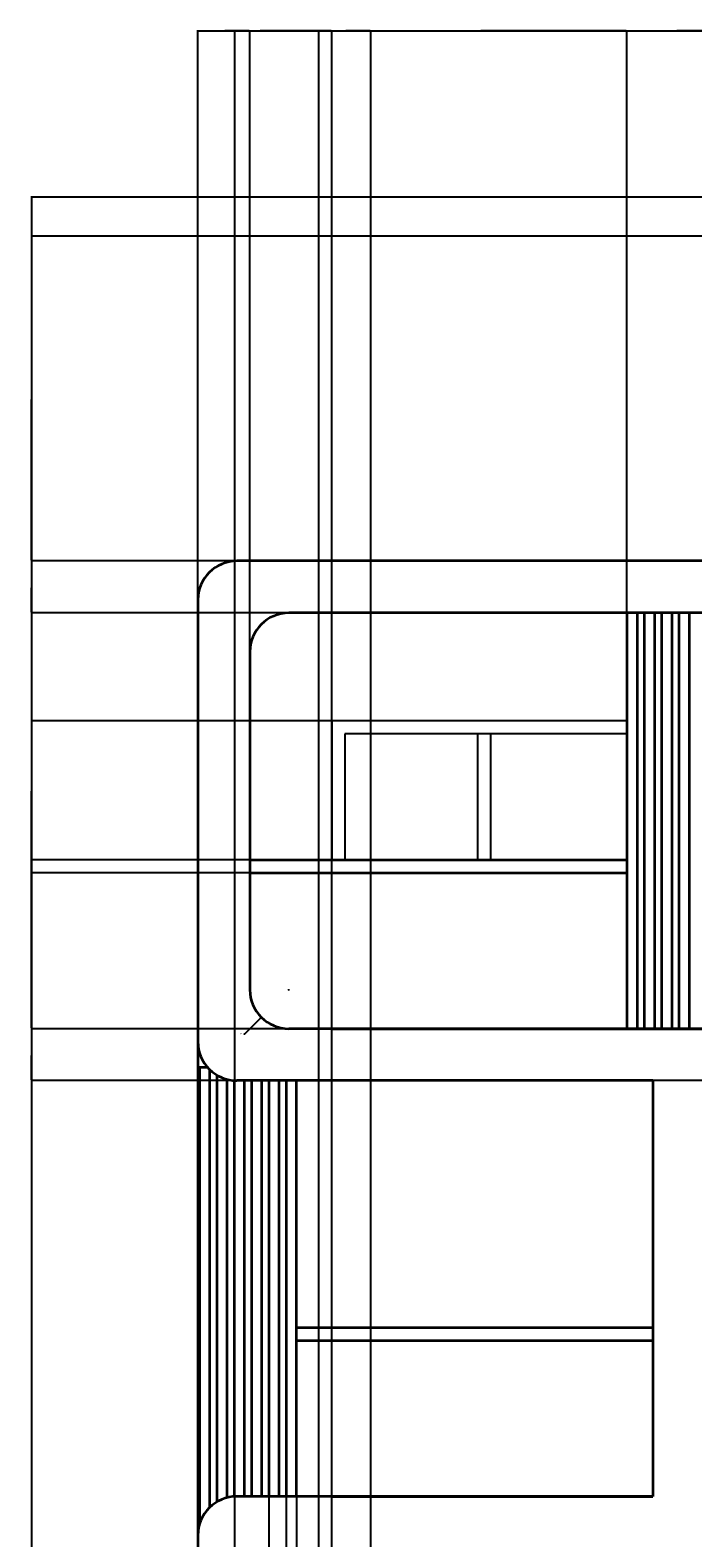
# Model space of a CAD drawing. Units: inches. Extents: x -15 to 605, y -220 to 570.
# Tile 7 of 10: x -15 to 138, y 222 to 570. Entities that reach past the tile are written whole.
import ezdxf

# ---------------------------------------------------------------- set-up
doc = ezdxf.new("R2010")
doc.units = ezdxf.units.IN
doc.header["$MEASUREMENT"] = 0
for name, color, linetype, lineweight in [('A-ANNO-DIMS', 2, 'Continuous', 18), ('A-ELEV', 7, 'Continuous', 35), ('A-GLAZ', 4, 'Continuous', 25)]:
    doc.layers.add(name, color=color, linetype=linetype, lineweight=lineweight)
doc.styles.get("Standard").update_dxf_attribs({"font": 'arial.ttf'})
doc.dimstyles.get("Standard").update_dxf_attribs({"dimtxt": 0.18, "dimasz": 0.18, "dimexe": 0.18, "dimexo": 0.0625, "dimgap": 0.09, "dimtad": 0, "dimtih": 1, "dimtoh": 1, "dimdec": 4, "dimzin": 0, "dimdsep": 46, "dimtxsty": 'Standard', "dimcen": 0.09, "dimadec": 0, "dimazin": 0, "dimtfac": 1, "dimtdec": 4, "dimtofl": 0, "dimtmove": 0, "dimatfit": 3, "dimfxl": 1, "dimtolj": 1, "dimtzin": 0, "dimarcsym": 0})

# ---------------------------------------------------------------- blocks, each defined once
blk = doc.blocks.new('*D8')
at = {"layer": 'A-ANNO-DIMS', "color": 0, "lineweight": -2, "transparency": 16777216}
for p, q in [((23.99, 3.88), (23.99, 570.4)), ((24.17, 570.22), (263.7, 570.22)), ((503.81, 570.22), (264.28, 570.22)), ((503.99, 531.88), (503.99, 570.4))]:
    blk.add_line(p, q, dxfattribs=at)
at = {"layer": 'A-ANNO-DIMS', "color": 0, "transparency": 16777216}
for points in [[(24.17, 570.25), (24.17, 570.19), (23.99, 570.22)], [(503.81, 570.25), (503.81, 570.19), (503.99, 570.22)]]:
    blk.add_solid(points, dxfattribs=at)
at = {"layer": 'Defpoints', "color": 0, "transparency": 16777216}
for p in [(503.99, 570.22), (503.99, 531.82), (23.99, 3.82)]:
    blk.add_point(p, dxfattribs=at)
at = {"layer": 'A-ANNO-DIMS', "color": 0, "transparency": 16777216, "insert": (263.99, 570.22), "char_height": 0.18, "attachment_point": 5}
blk.add_mtext('\\A1;480', dxfattribs=at)
blk = doc.blocks.new('*D9')
at = {"layer": 'A-ANNO-DIMS', "color": 0, "lineweight": -2, "transparency": 16777216}
for p, q in [((503.92, 531.82), (-14.59, 531.82)), ((-14.41, 531.64), (-14.41, 208)), ((-14.41, -116), (-14.41, 207.64)), ((23.92, -116.18), (-14.59, -116.18))]:
    blk.add_line(p, q, dxfattribs=at)
at = {"layer": 'A-ANNO-DIMS', "color": 0, "transparency": 16777216}
for points in [[(-14.44, 531.64), (-14.38, 531.64), (-14.41, 531.82)], [(-14.44, -116), (-14.38, -116), (-14.41, -116.18)]]:
    blk.add_solid(points, dxfattribs=at)
at = {"layer": 'Defpoints', "color": 0, "transparency": 16777216}
for p in [(-14.41, 531.82), (503.99, 531.82), (23.99, -116.18)]:
    blk.add_point(p, dxfattribs=at)
at = {"layer": 'A-ANNO-DIMS', "color": 0, "transparency": 16777216, "insert": (-14.41, 207.82), "char_height": 0.18, "attachment_point": 5}
blk.add_mtext('\\A1;648', dxfattribs=at)
blk = doc.blocks.new('*D18')
at = {"layer": 'A-ANNO-DIMS', "color": 0, "lineweight": -2, "transparency": 16777216}
for p, q in [((23.99, 3.88), (23.99, 570.4)), ((24.17, 570.22), (143.44, 570.22)), ((263.64, 570.22), (144.37, 570.22)), ((263.82, 447.88), (263.82, 570.4))]:
    blk.add_line(p, q, dxfattribs=at)
at = {"layer": 'A-ANNO-DIMS', "color": 0, "transparency": 16777216}
for points in [[(24.17, 570.25), (24.17, 570.19), (23.99, 570.22)], [(263.64, 570.25), (263.64, 570.19), (263.82, 570.22)]]:
    blk.add_solid(points, dxfattribs=at)
at = {"layer": 'Defpoints', "color": 0, "transparency": 16777216}
for p in [(263.82, 570.22), (263.82, 447.82), (23.99, 3.82)]:
    blk.add_point(p, dxfattribs=at)
at = {"layer": 'A-ANNO-DIMS', "color": 0, "transparency": 16777216, "insert": (143.9, 570.22), "char_height": 0.18, "attachment_point": 5}
blk.add_mtext('\\A1;239.83', dxfattribs=at)
blk = doc.blocks.new('*D52')
at = {"layer": 'A-ANNO-DIMS', "color": 0, "lineweight": -2, "transparency": 16777216}
for p, q in [((23.99, -32.12), (23.99, 570.4)), ((24.17, 570.22), (37.55, 570.22)), ((51.73, 570.22), (38.34, 570.22)), ((51.91, -32.12), (51.91, 570.4))]:
    blk.add_line(p, q, dxfattribs=at)
at = {"layer": 'A-ANNO-DIMS', "color": 0, "transparency": 16777216}
for points in [[(24.17, 570.25), (24.17, 570.19), (23.99, 570.22)], [(51.73, 570.25), (51.73, 570.19), (51.91, 570.22)]]:
    blk.add_solid(points, dxfattribs=at)
at = {"layer": 'Defpoints', "color": 0, "transparency": 16777216}
for p in [(51.91, 570.22), (23.99, -32.18), (51.91, -32.18)]:
    blk.add_point(p, dxfattribs=at)
at = {"layer": 'A-ANNO-DIMS', "color": 0, "transparency": 16777216, "insert": (37.95, 570.22), "char_height": 0.18, "attachment_point": 5}
blk.add_mtext('\\A1;27.92', dxfattribs=at)
blk = doc.blocks.new('*D53')
at = {"layer": 'A-ANNO-DIMS', "color": 0, "lineweight": -2, "transparency": 16777216}
for p, q in [((51.91, -32.12), (51.91, 570.4)), ((52.09, 570.22), (57.7, 570.22)), ((63.73, 570.22), (58.12, 570.22)), ((63.91, -32.12), (63.91, 570.4))]:
    blk.add_line(p, q, dxfattribs=at)
at = {"layer": 'A-ANNO-DIMS', "color": 0, "transparency": 16777216}
for points in [[(52.09, 570.25), (52.09, 570.19), (51.91, 570.22)], [(63.73, 570.25), (63.73, 570.19), (63.91, 570.22)]]:
    blk.add_solid(points, dxfattribs=at)
at = {"layer": 'Defpoints', "color": 0, "transparency": 16777216}
for p in [(63.91, 570.22), (51.91, -32.18), (63.91, -32.18)]:
    blk.add_point(p, dxfattribs=at)
at = {"layer": 'A-ANNO-DIMS', "color": 0, "transparency": 16777216, "insert": (57.91, 570.22), "char_height": 0.18, "attachment_point": 5}
blk.add_mtext('\\A1;12', dxfattribs=at)
blk = doc.blocks.new('*D54')
at = {"layer": 'A-ANNO-DIMS', "color": 0, "lineweight": -2, "transparency": 16777216}
for p, q in [((63.91, -32.12), (63.91, 570.4)), ((64.09, 570.22), (142.07, 570.22)), ((220.96, 570.22), (142.98, 570.22)), ((221.14, -31.58), (221.14, 570.4))]:
    blk.add_line(p, q, dxfattribs=at)
at = {"layer": 'A-ANNO-DIMS', "color": 0, "transparency": 16777216}
for points in [[(64.09, 570.25), (64.09, 570.19), (63.91, 570.22)], [(220.96, 570.25), (220.96, 570.19), (221.14, 570.22)]]:
    blk.add_solid(points, dxfattribs=at)
at = {"layer": 'Defpoints', "color": 0, "transparency": 16777216}
for p in [(221.14, 570.22), (63.91, -32.18), (221.14, -31.64)]:
    blk.add_point(p, dxfattribs=at)
at = {"layer": 'A-ANNO-DIMS', "color": 0, "transparency": 16777216, "insert": (142.53, 570.22), "char_height": 0.18, "attachment_point": 5}
blk.add_mtext('\\A1;157.24', dxfattribs=at)
blk = doc.blocks.new('*D74')
at = {"layer": 'A-ANNO-DIMS', "color": 0, "lineweight": -2, "transparency": 16777216}
for p, q in [((272.75, 522.82), (-14.59, 522.82)), ((-14.41, 522.64), (-14.41, 485.5)), ((-14.41, 448), (-14.41, 485.14)), ((272.75, 447.82), (-14.59, 447.82))]:
    blk.add_line(p, q, dxfattribs=at)
at = {"layer": 'A-ANNO-DIMS', "color": 0, "transparency": 16777216}
for points in [[(-14.44, 522.64), (-14.38, 522.64), (-14.41, 522.82)], [(-14.44, 448), (-14.38, 448), (-14.41, 447.82)]]:
    blk.add_solid(points, dxfattribs=at)
at = {"layer": 'Defpoints', "color": 0, "transparency": 16777216}
for p in [(-14.41, 522.82), (272.82, 522.82), (272.82, 447.82)]:
    blk.add_point(p, dxfattribs=at)
at = {"layer": 'A-ANNO-DIMS', "color": 0, "transparency": 16777216, "insert": (-14.41, 485.32), "char_height": 0.18, "attachment_point": 5}
blk.add_mtext('\\A1;75', dxfattribs=at)
blk = doc.blocks.new('*D76')
at = {"layer": 'A-ANNO-DIMS', "color": 0, "lineweight": -2, "transparency": 16777216}
for p, q in [((272.92, 339.82), (-14.59, 339.82)), ((-14.41, 339.64), (-14.41, 334)), ((-14.41, 328), (-14.41, 333.64)), ((272.92, 327.82), (-14.59, 327.82))]:
    blk.add_line(p, q, dxfattribs=at)
at = {"layer": 'A-ANNO-DIMS', "color": 0, "transparency": 16777216}
for points in [[(-14.44, 339.64), (-14.38, 339.64), (-14.41, 339.82)], [(-14.44, 328), (-14.38, 328), (-14.41, 327.82)]]:
    blk.add_solid(points, dxfattribs=at)
at = {"layer": 'Defpoints', "color": 0, "transparency": 16777216}
for p in [(-14.41, 339.82), (272.99, 339.82), (272.99, 327.82)]:
    blk.add_point(p, dxfattribs=at)
at = {"layer": 'A-ANNO-DIMS', "color": 0, "transparency": 16777216, "insert": (-14.41, 333.82), "char_height": 0.18, "attachment_point": 5}
blk.add_mtext('\\A1;12', dxfattribs=at)
blk = doc.blocks.new('*D77')
at = {"layer": 'A-ANNO-DIMS', "color": 0, "lineweight": -2, "transparency": 16777216}
for p, q in [((272.92, 435.82), (-14.59, 435.82)), ((-14.41, 435.64), (-14.41, 388)), ((-14.41, 340), (-14.41, 387.64)), ((272.92, 339.82), (-14.59, 339.82))]:
    blk.add_line(p, q, dxfattribs=at)
at = {"layer": 'A-ANNO-DIMS', "color": 0, "transparency": 16777216}
for points in [[(-14.44, 435.64), (-14.38, 435.64), (-14.41, 435.82)], [(-14.44, 340), (-14.38, 340), (-14.41, 339.82)]]:
    blk.add_solid(points, dxfattribs=at)
at = {"layer": 'Defpoints', "color": 0, "transparency": 16777216}
for p in [(-14.41, 435.82), (272.99, 435.82), (272.99, 339.82)]:
    blk.add_point(p, dxfattribs=at)
at = {"layer": 'A-ANNO-DIMS', "color": 0, "transparency": 16777216, "insert": (-14.41, 387.82), "char_height": 0.18, "attachment_point": 5}
blk.add_mtext('\\A1;96', dxfattribs=at)
blk = doc.blocks.new('*D78')
at = {"layer": 'A-ANNO-DIMS', "color": 0, "lineweight": -2, "transparency": 16777216}
for p, q in [((272.75, 447.82), (-14.59, 447.82)), ((-14.41, 447.64), (-14.41, 442)), ((-14.41, 436), (-14.41, 441.64)), ((272.92, 435.82), (-14.59, 435.82))]:
    blk.add_line(p, q, dxfattribs=at)
at = {"layer": 'A-ANNO-DIMS', "color": 0, "transparency": 16777216}
for points in [[(-14.44, 447.64), (-14.38, 447.64), (-14.41, 447.82)], [(-14.44, 436), (-14.38, 436), (-14.41, 435.82)]]:
    blk.add_solid(points, dxfattribs=at)
at = {"layer": 'Defpoints', "color": 0, "transparency": 16777216}
for p in [(-14.41, 447.82), (272.82, 447.82), (272.99, 435.82)]:
    blk.add_point(p, dxfattribs=at)
at = {"layer": 'A-ANNO-DIMS', "color": 0, "transparency": 16777216, "insert": (-14.41, 441.82), "char_height": 0.18, "attachment_point": 5}
blk.add_mtext('\\A1;12', dxfattribs=at)
blk = doc.blocks.new('*D79')
at = {"layer": 'A-ANNO-DIMS', "color": 0, "lineweight": -2, "transparency": 16777216}
for p, q in [((23.99, 336.88), (23.99, 570.4)), ((24.17, 570.22), (29.78, 570.22)), ((35.81, 570.22), (30.2, 570.22)), ((35.99, 348.88), (35.99, 570.4))]:
    blk.add_line(p, q, dxfattribs=at)
at = {"layer": 'A-ANNO-DIMS', "color": 0, "transparency": 16777216}
for points in [[(24.17, 570.25), (24.17, 570.19), (23.99, 570.22)], [(35.81, 570.25), (35.81, 570.19), (35.99, 570.22)]]:
    blk.add_solid(points, dxfattribs=at)
at = {"layer": 'Defpoints', "color": 0, "transparency": 16777216}
for p in [(35.99, 570.22), (35.99, 348.82), (23.99, 336.82)]:
    blk.add_point(p, dxfattribs=at)
at = {"layer": 'A-ANNO-DIMS', "color": 0, "transparency": 16777216, "insert": (29.99, 570.22), "char_height": 0.18, "attachment_point": 5}
blk.add_mtext('\\A1;12', dxfattribs=at)
blk = doc.blocks.new('*D80')
at = {"layer": 'A-ANNO-DIMS', "color": 0, "lineweight": -2, "transparency": 16777216}
for p, q in [((35.99, 348.88), (35.99, 570.4)), ((36.17, 570.22), (45.01, 570.22)), ((54.75, 570.22), (45.92, 570.22)), ((54.93, 378.88), (54.93, 570.4))]:
    blk.add_line(p, q, dxfattribs=at)
at = {"layer": 'A-ANNO-DIMS', "color": 0, "transparency": 16777216}
for points in [[(36.17, 570.25), (36.17, 570.19), (35.99, 570.22)], [(54.75, 570.25), (54.75, 570.19), (54.93, 570.22)]]:
    blk.add_solid(points, dxfattribs=at)
at = {"layer": 'Defpoints', "color": 0, "transparency": 16777216}
for p in [(54.93, 570.22), (54.93, 378.82), (35.99, 348.82)]:
    blk.add_point(p, dxfattribs=at)
at = {"layer": 'A-ANNO-DIMS', "color": 0, "transparency": 16777216, "insert": (45.46, 570.22), "char_height": 0.18, "attachment_point": 5}
blk.add_mtext('\\A1;18.946', dxfattribs=at)
blk = doc.blocks.new('*D81')
at = {"layer": 'A-ANNO-DIMS', "color": 0, "lineweight": -2, "transparency": 16777216}
for p, q in [((54.93, 378.88), (54.93, 570.4)), ((55.11, 570.22), (88.67, 570.22)), ((122.85, 570.22), (89.29, 570.22)), ((123.03, 339.88), (123.03, 570.4))]:
    blk.add_line(p, q, dxfattribs=at)
at = {"layer": 'A-ANNO-DIMS', "color": 0, "transparency": 16777216}
for points in [[(55.11, 570.25), (55.11, 570.19), (54.93, 570.22)], [(122.85, 570.25), (122.85, 570.19), (123.03, 570.22)]]:
    blk.add_solid(points, dxfattribs=at)
at = {"layer": 'Defpoints', "color": 0, "transparency": 16777216}
for p in [(123.03, 570.22), (54.93, 378.82), (123.03, 339.82)]:
    blk.add_point(p, dxfattribs=at)
at = {"layer": 'A-ANNO-DIMS', "color": 0, "transparency": 16777216, "insert": (88.98, 570.22), "char_height": 0.18, "attachment_point": 5}
blk.add_mtext('\\A1;68.1', dxfattribs=at)
blk = doc.blocks.new('*D82')
at = {"layer": 'A-ANNO-DIMS', "color": 0, "lineweight": -2, "transparency": 16777216}
for p, q in [((123.03, 339.88), (123.03, 570.4)), ((123.21, 570.22), (133.9, 570.22)), ((145.25, 570.22), (134.55, 570.22)), ((145.43, 339.88), (145.43, 570.4))]:
    blk.add_line(p, q, dxfattribs=at)
at = {"layer": 'A-ANNO-DIMS', "color": 0, "transparency": 16777216}
for points in [[(123.21, 570.25), (123.21, 570.19), (123.03, 570.22)], [(145.25, 570.25), (145.25, 570.19), (145.43, 570.22)]]:
    blk.add_solid(points, dxfattribs=at)
at = {"layer": 'Defpoints', "color": 0, "transparency": 16777216}
for p in [(145.43, 570.22), (123.03, 339.82), (145.43, 339.82)]:
    blk.add_point(p, dxfattribs=at)
at = {"layer": 'A-ANNO-DIMS', "color": 0, "transparency": 16777216, "insert": (134.23, 570.22), "char_height": 0.18, "attachment_point": 5}
blk.add_mtext('\\A1;22.4', dxfattribs=at)
blk = doc.blocks.new('*D96')
at = {"layer": 'A-ANNO-DIMS', "color": 0, "lineweight": -2, "transparency": 16777216}
for p, q in [((54.87, 410.89), (-14.59, 410.89)), ((-14.41, 410.71), (-14.41, 395.04)), ((-14.41, 379), (-14.41, 394.67)), ((54.87, 378.82), (-14.59, 378.82))]:
    blk.add_line(p, q, dxfattribs=at)
at = {"layer": 'A-ANNO-DIMS', "color": 0, "transparency": 16777216}
for points in [[(-14.44, 410.71), (-14.38, 410.71), (-14.41, 410.89)], [(-14.44, 379), (-14.38, 379), (-14.41, 378.82)]]:
    blk.add_solid(points, dxfattribs=at)
at = {"layer": 'Defpoints', "color": 0, "transparency": 16777216}
for p in [(-14.41, 410.89), (54.93, 410.89), (54.93, 378.82)]:
    blk.add_point(p, dxfattribs=at)
at = {"layer": 'A-ANNO-DIMS', "color": 0, "transparency": 16777216, "insert": (-14.41, 394.85), "char_height": 0.18, "attachment_point": 5}
blk.add_mtext('\\A1;32.07', dxfattribs=at)
blk = doc.blocks.new('*D97')
at = {"layer": 'A-ANNO-DIMS', "color": 0, "lineweight": -2, "transparency": 16777216}
for p, q in [((122.96, 375.82), (-14.59, 375.82)), ((-14.41, 375.64), (-14.41, 358)), ((-14.41, 340), (-14.41, 357.64)), ((122.96, 339.82), (-14.59, 339.82))]:
    blk.add_line(p, q, dxfattribs=at)
at = {"layer": 'A-ANNO-DIMS', "color": 0, "transparency": 16777216}
for points in [[(-14.44, 375.64), (-14.38, 375.64), (-14.41, 375.82)], [(-14.44, 340), (-14.38, 340), (-14.41, 339.82)]]:
    blk.add_solid(points, dxfattribs=at)
at = {"layer": 'Defpoints', "color": 0, "transparency": 16777216}
for p in [(-14.41, 375.82), (123.03, 375.82), (123.03, 339.82)]:
    blk.add_point(p, dxfattribs=at)
at = {"layer": 'A-ANNO-DIMS', "color": 0, "transparency": 16777216, "insert": (-14.41, 357.82), "char_height": 0.18, "attachment_point": 5}
blk.add_mtext('\\A1;36', dxfattribs=at)
blk = doc.blocks.new('*D110')
at = {"layer": 'A-ANNO-DIMS', "color": 0, "lineweight": -2, "transparency": 16777216}
for p, q in [((32.53, 115.18), (32.53, 570.4)), ((32.71, 570.22), (43.34, 570.22)), ((54.75, 570.22), (44.13, 570.22)), ((54.93, 115.18), (54.93, 570.4))]:
    blk.add_line(p, q, dxfattribs=at)
at = {"layer": 'A-ANNO-DIMS', "color": 0, "transparency": 16777216}
for points in [[(32.71, 570.25), (32.71, 570.19), (32.53, 570.22)], [(54.75, 570.25), (54.75, 570.19), (54.93, 570.22)]]:
    blk.add_solid(points, dxfattribs=at)
at = {"layer": 'Defpoints', "color": 0, "transparency": 16777216}
for p in [(54.93, 570.22), (32.53, 115.12), (54.93, 115.12)]:
    blk.add_point(p, dxfattribs=at)
at = {"layer": 'A-ANNO-DIMS', "color": 0, "transparency": 16777216, "insert": (43.73, 570.22), "char_height": 0.18, "attachment_point": 5}
blk.add_mtext('\\A1;22.40', dxfattribs=at)
blk = doc.blocks.new('*D113')
at = {"layer": 'A-ANNO-DIMS', "color": 0, "lineweight": -2, "transparency": 16777216}
for p, q in [((44.35, 231.76), (44.35, -154.76)), ((46.75, 231.76), (46.75, -154.76)), ((44.53, -154.58), (45.23, -154.58)), ((46.57, -154.58), (45.88, -154.58))]:
    blk.add_line(p, q, dxfattribs=at)
at = {"layer": 'A-ANNO-DIMS', "color": 0, "transparency": 16777216}
for points in [[(44.53, -154.55), (44.53, -154.61), (44.35, -154.58)], [(46.57, -154.55), (46.57, -154.61), (46.75, -154.58)]]:
    blk.add_solid(points, dxfattribs=at)
at = {"layer": 'Defpoints', "color": 0, "transparency": 16777216}
for p in [(44.35, 231.82), (46.75, 231.82), (46.75, -154.58)]:
    blk.add_point(p, dxfattribs=at)
at = {"layer": 'A-ANNO-DIMS', "color": 0, "transparency": 16777216, "insert": (45.55, -154.58), "char_height": 0.18, "attachment_point": 5}
blk.add_mtext('\\A1;2.40', dxfattribs=at)
blk = doc.blocks.new('*D114')
at = {"layer": 'A-ANNO-DIMS', "color": 0, "lineweight": -2, "transparency": 16777216}
for p, q in [((40.35, 231.76), (40.35, -154.76)), ((44.35, 231.76), (44.35, -154.76)), ((40.53, -154.58), (42.03, -154.58)), ((44.17, -154.58), (42.68, -154.58))]:
    blk.add_line(p, q, dxfattribs=at)
at = {"layer": 'A-ANNO-DIMS', "color": 0, "transparency": 16777216}
for points in [[(40.53, -154.55), (40.53, -154.61), (40.35, -154.58)], [(44.17, -154.55), (44.17, -154.61), (44.35, -154.58)]]:
    blk.add_solid(points, dxfattribs=at)
at = {"layer": 'Defpoints', "color": 0, "transparency": 16777216}
for p in [(40.35, 231.82), (44.35, 231.82), (44.35, -154.58)]:
    blk.add_point(p, dxfattribs=at)
at = {"layer": 'A-ANNO-DIMS', "color": 0, "transparency": 16777216, "insert": (42.35, -154.58), "char_height": 0.18, "attachment_point": 5}
blk.add_mtext('\\A1;4.00', dxfattribs=at)
blk = doc.blocks.new('*D121')
at = {"layer": 'A-ANNO-DIMS', "color": 0, "lineweight": -2, "transparency": 16777216}
for p, q in [((44.9, 348.82), (45.08, 348.82)), ((44.99, 348.73), (44.99, 348.91)), ((34.8, 338.64), (38.5, 342.33)), ((34.62, 338.64), (34.8, 338.64))]:
    blk.add_line(p, q, dxfattribs=at)
at = {"layer": 'A-ANNO-DIMS', "color": 0, "transparency": 16777216}
blk.add_solid([(38.47, 342.35), (38.52, 342.31), (38.62, 342.46)], dxfattribs=at)
at = {"layer": 'Defpoints', "color": 0, "transparency": 16777216}
for p in [(44.99, 348.82), (38.62, 342.46)]:
    blk.add_point(p, dxfattribs=at)
at = {"layer": 'A-ANNO-DIMS', "color": 0, "transparency": 16777216, "insert": (34.02, 338.64), "char_height": 0.18, "attachment_point": 5}
blk.add_mtext('\\A1;4X R9.00', dxfattribs=at)

msp = doc.modelspace()

# ---------------------------------------------------------------- linework, layer by layer
at = {"layer": 'A-ELEV'}
for p, q in [((263.8163, 447.8187), (32.9872, 447.8187)), ((23.9872, 438.8187), (23.9872, 339.8187)), ((23.9872, 438.8187), (23.9872, 336.8187)), ((373.1921, 435.8187), (44.9872, 435.8187)), ((35.9872, 426.8187), (35.9872, 348.8187)), ((23.9872, 339.8187), (23.9872, 327.8187)), ((373.1921, 339.8187), (44.9872, 339.8187)), ((54.933, 339.8187), (212.3003, 339.8187)), ((26.259, 330.8412), (24.3536, 330.8412)), ((24.3536, 330.8412), (24.3536, 225.3603)), ((23.9872, 327.8187), (24.3536, 327.8187)), ((26.7536, 229.3104), (26.7536, 330.327)), ((128.9872, 327.8187), (32.9872, 327.8187)), ((128.9872, 327.8187), (128.9872, 231.8187)), ((128.9872, 231.8187), (32.9872, 231.8187)), ((54.933, 231.8187), (128.9872, 231.8187))]:
    msp.add_line(p, q, dxfattribs=at)
for points in [[(123.0266, 435.8187), (123.0266, 339.8187), (125.4266, 339.8187), (125.4266, 435.8187)], [(127.0267, 435.8187), (127.0267, 339.8187), (129.4268, 339.8187), (129.4268, 435.8187)], [(131.0268, 435.8187), (131.0268, 339.8187), (133.4269, 339.8187), (133.4269, 435.8187)], [(135.0269, 435.8187), (135.0269, 339.8187), (137.427, 339.8187), (137.427, 435.8187)], [(35.9872, 378.8187), (74.3396, 378.8187), (123.0266, 378.8187)], [(35.9872, 375.8187), (74.3396, 375.8187), (123.0266, 375.8187)], [(28.3537, 329.1031), (28.3537, 230.5343)], [(30.7538, 231.5372), (30.7538, 328.1003)], [(32.3538, 327.841), (32.3538, 231.7964)], [(34.7539, 231.8187), (34.7539, 327.8187)], [(36.3539, 327.8187), (36.3539, 231.8187)], [(38.754, 231.8187), (38.754, 327.8187)], [(40.354, 327.8187), (40.354, 231.8187)], [(42.7541, 231.8187), (42.7541, 327.8187)], [(44.3542, 327.8187), (44.3542, 231.8187)], [(46.7542, 231.8187), (46.7542, 327.8187)], [(46.7542, 270.8187), (128.9872, 270.8187)], [(46.7542, 267.8187), (128.9872, 267.8187)]]:
    msp.add_lwpolyline(points, dxfattribs=at)
msp.add_lwpolyline([(23.9872, 222.8187), (23.9872, 120.8187, 0.41421356), (32.9872, 111.8187)], format="xyb", dxfattribs=at)
for centre, start, end in [((32.9872, 438.8187), 90, 180), ((44.9872, 426.8187), 90, 180), ((44.9872, 348.8187), 180, 270), ((32.9872, 336.8187), 180, 270), ((32.9872, 222.8187), 90, 180)]:
    msp.add_arc(centre, 9, start, end, dxfattribs=at)
at = {"layer": 'A-GLAZ'}
for p, q in [((123.0266, 410.8893), (54.933, 410.8893)), ((54.933, 410.8893), (54.933, 378.8187)), ((123.0266, 407.8893), (57.933, 407.8893)), ((57.933, 407.8893), (57.933, 378.8187)), ((88.549, 407.8893), (88.549, 378.8187)), ((91.549, 407.8893), (91.549, 378.8187))]:
    msp.add_line(p, q, dxfattribs=at)

# ---------------------------------------------------------------- dimensions: what is measured, and where the dimension line sits
at = {"layer": 'A-ANNO-DIMS'}
for base, p1, p2, override, picture, middle in [((503.9872, 570.2187), (23.9872, 3.8187), (503.9872, 531.8187), {"dimdec": 0, "dimlfac": 1, "dimrnd": 0, "dimzin": 0, "dimdsep": 46, "dimlunit": 2}, '*D8', (263.9872, 570.2187)), ((263.8163, 570.2187), (23.9872, 3.8187), (263.8163, 447.8187), {"dimdec": 2, "dimlfac": 1, "dimrnd": 0, "dimzin": 0, "dimdsep": 46, "dimlunit": 2}, '*D18', (143.9018, 570.2187)), ((51.9067, 570.2187), (23.9872, -32.1813), (51.9067, -32.1813), {"dimdec": 2, "dimlfac": 1, "dimrnd": 0, "dimzin": 0, "dimdsep": 46, "dimlunit": 2}, '*D52', (37.947, 570.2187)), ((35.9872, 570.2187), (23.9872, 336.8187), (35.9872, 348.8187), {"dimdec": 0, "dimlfac": 1, "dimrnd": 0, "dimzin": 0, "dimdsep": 46, "dimlunit": 2}, '*D79', (29.9872, 570.2187)), ((54.933, 570.2187), (32.5323, 115.1203), (54.933, 115.1203), {"dimdec": 2, "dimlfac": 1, "dimrnd": 0, "dimzin": 0, "dimdsep": 46, "dimlunit": 2}, '*D110', (43.7326, 570.2187)), ((54.933, 570.2187), (35.9872, 348.8187), (54.933, 378.8187), {"dimdec": 3, "dimlfac": 1, "dimrnd": 0, "dimzin": 0, "dimdsep": 46, "dimlunit": 2}, '*D80', (45.4601, 570.2187)), ((63.9067, 570.2187), (51.9067, -32.1813), (63.9067, -32.1813), {"dimdec": 0, "dimlfac": 1, "dimrnd": 0, "dimzin": 0, "dimdsep": 46, "dimlunit": 2}, '*D53', (57.9067, 570.2187)), ((123.0266, 570.2187), (54.933, 378.8187), (123.0266, 339.8187), {"dimdec": 1, "dimlfac": 1, "dimrnd": 0, "dimzin": 0, "dimdsep": 46, "dimlunit": 2}, '*D81', (88.9798, 570.2187)), ((221.1439, 570.2187), (63.9067, -32.1813), (221.1439, -31.6396), {"dimdec": 2, "dimlfac": 1, "dimrnd": 0, "dimzin": 0, "dimdsep": 46, "dimlunit": 2}, '*D54', (142.5253, 570.2187)), ((145.4272, 570.2187), (123.0266, 339.8187), (145.4272, 339.8187), {"dimdec": 1, "dimlfac": 1, "dimrnd": 0, "dimzin": 0, "dimdsep": 46, "dimlunit": 2}, '*D82', (134.2269, 570.2187)), ((44.3542, -154.5813), (40.354, 231.8187), (44.3542, 231.8187), {"dimdec": 2, "dimlfac": 1, "dimrnd": 0, "dimzin": 0, "dimdsep": 46, "dimlunit": 2}, '*D114', (42.3541, -154.5813)), ((46.7542, -154.5813), (44.3542, 231.8187), (46.7542, 231.8187), {"dimdec": 2, "dimlfac": 1, "dimrnd": 0, "dimzin": 0, "dimdsep": 46, "dimlunit": 2}, '*D113', (45.5542, -154.5813))]:
    dim = msp.add_linear_dim(base=base, p1=p1, p2=p2, dimstyle='Standard', override=override, dxfattribs=at)
    dim.commit()
    dim.dimension.update_dxf_attribs({"geometry": picture, "text_midpoint": middle})
for base, p1, p2, override, picture, middle in [((-14.4128, 531.8187), (23.9872, -116.1813), (503.9872, 531.8187), {"dimdec": 0, "dimlfac": 1, "dimrnd": 0, "dimzin": 0, "dimdsep": 46, "dimlunit": 2}, '*D9', (-14.4128, 207.8187)), ((-14.4128, 522.8187), (272.8163, 447.8187), (272.8163, 522.8187), {"dimdec": 0, "dimlfac": 1, "dimrnd": 0, "dimzin": 0, "dimdsep": 46, "dimlunit": 2}, '*D74', (-14.4128, 485.3187)), ((-14.4128, 447.8187), (272.9872, 435.8187), (272.8163, 447.8187), {"dimdec": 0, "dimlfac": 1, "dimrnd": 0, "dimzin": 0, "dimdsep": 46, "dimlunit": 2}, '*D78', (-14.4128, 441.8187)), ((-14.4128, 435.8187), (272.9872, 339.8187), (272.9872, 435.8187), {"dimdec": 0, "dimlfac": 1, "dimrnd": 0, "dimzin": 0, "dimdsep": 46, "dimlunit": 2}, '*D77', (-14.4128, 387.8187)), ((-14.4128, 410.8893), (54.933, 378.8187), (54.933, 410.8893), {"dimdec": 2, "dimlfac": 1, "dimrnd": 0, "dimzin": 0, "dimdsep": 46, "dimlunit": 2}, '*D96', (-14.4128, 394.854)), ((-14.4128, 375.8187), (123.0266, 339.8187), (123.0266, 375.8187), {"dimdec": 0, "dimlfac": 1, "dimrnd": 0, "dimzin": 0, "dimdsep": 46, "dimlunit": 2}, '*D97', (-14.4128, 357.8187)), ((-14.4128, 339.8187), (272.9872, 327.8187), (272.9872, 339.8187), {"dimdec": 0, "dimlfac": 1, "dimrnd": 0, "dimzin": 0, "dimdsep": 46, "dimlunit": 2}, '*D76', (-14.4128, 333.8187))]:
    dim = msp.add_linear_dim(base=base, p1=p1, p2=p2, angle=90, dimstyle='Standard', override=override, dxfattribs=at)
    dim.commit()
    dim.dimension.update_dxf_attribs({"geometry": picture, "text_midpoint": middle})
dim = msp.add_radius_dim(center=(44.9872, 348.8187), mpoint=(38.623, 342.455), text='4X <>', dimstyle='Standard', override={"dimdec": 2, "dimlfac": 1, "dimrnd": 0, "dimzin": 0, "dimdsep": 46, "dimlunit": 2}, dxfattribs=at)
dim.commit()
dim.dimension.update_dxf_attribs({"geometry": '*D121', "text_midpoint": (34.0179, 338.6368), "dimtype": 164})

doc.saveas('drawing.dxf')
